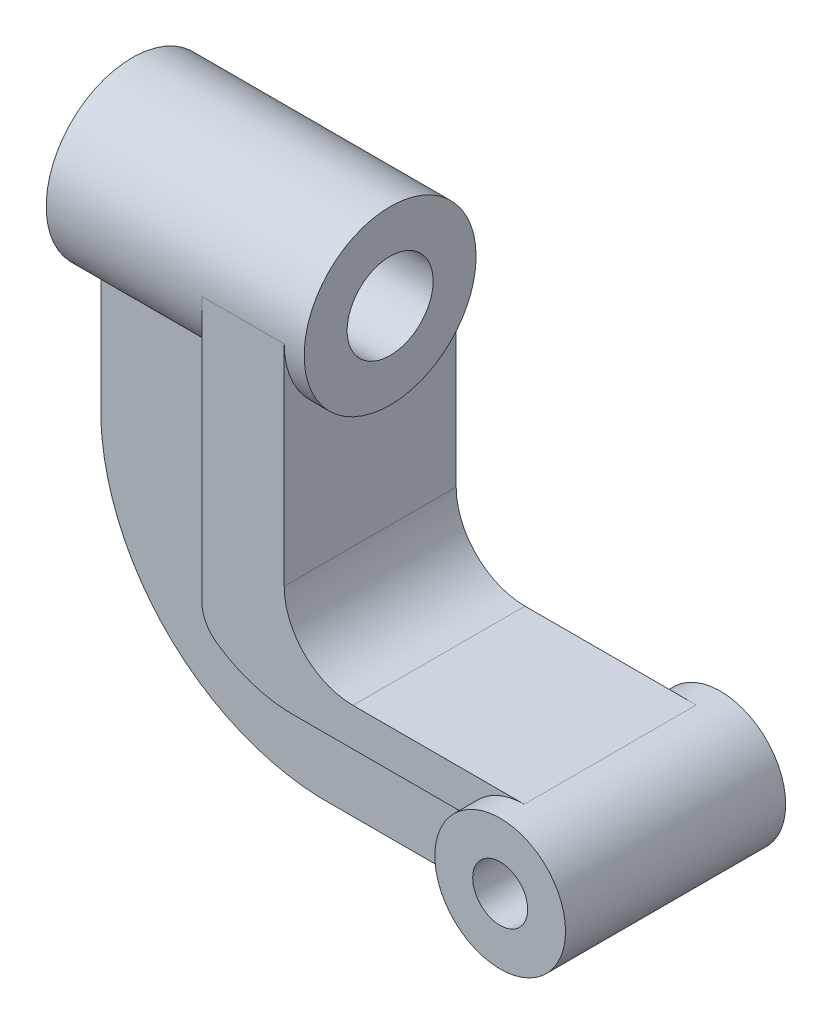
ISO-10303-21;
HEADER;
FILE_DESCRIPTION(('STEP AP214'),'2;1');
FILE_NAME('part.step','',(''),(''),'','','');
FILE_SCHEMA(('AUTOMOTIVE_DESIGN { 1 0 10303 214 1 1 1 1 }'));
ENDSEC;
DATA;
#1=APPLICATION_CONTEXT('core data for automotive mechanical design processes');
#2=APPLICATION_PROTOCOL_DEFINITION('international standard','automotive_design',2000,#1);
#3=PRODUCT_CONTEXT('',#1,'mechanical');
#4=PRODUCT('Part','Part','',(#3));
#5=PRODUCT_RELATED_PRODUCT_CATEGORY('part','',(#4));
#6=PRODUCT_DEFINITION_FORMATION('','',#4);
#7=PRODUCT_DEFINITION_CONTEXT('part definition',#1,'design');
#8=PRODUCT_DEFINITION('design','',#6,#7);
#9=PRODUCT_DEFINITION_SHAPE('','',#8);
#10=(LENGTH_UNIT() NAMED_UNIT(*) SI_UNIT(.MILLI.,.METRE.));
#11=(NAMED_UNIT(*) PLANE_ANGLE_UNIT() SI_UNIT($,.RADIAN.));
#12=(NAMED_UNIT(*) SI_UNIT($,.STERADIAN.) SOLID_ANGLE_UNIT());
#13=UNCERTAINTY_MEASURE_WITH_UNIT(LENGTH_MEASURE(1.E-05),#10,'distance_accuracy_value','');
#14=(GEOMETRIC_REPRESENTATION_CONTEXT(3) GLOBAL_UNCERTAINTY_ASSIGNED_CONTEXT((#13)) GLOBAL_UNIT_ASSIGNED_CONTEXT((#10,
#11,#12)) REPRESENTATION_CONTEXT('',''));
#15=CARTESIAN_POINT('',(0.,0.,0.));
#16=DIRECTION('',(0.,0.,1.));
#17=DIRECTION('',(1.,0.,0.));
#18=AXIS2_PLACEMENT_3D('',#15,#16,#17);
#19=CARTESIAN_POINT('',(37.5,0.,0.));
#20=DIRECTION('',(-1.,0.,0.));
#21=DIRECTION('',(0.,0.,1.));
#22=AXIS2_PLACEMENT_3D('',#19,#20,#21);
#23=CYLINDRICAL_SURFACE('',#22,25.);
#24=CARTESIAN_POINT('',(-37.5,0.,0.));
#25=DIRECTION('',(1.,0.,0.));
#26=DIRECTION('',(0.,0.,-1.));
#27=AXIS2_PLACEMENT_3D('',#24,#25,#26);
#28=CIRCLE('',#27,25.);
#29=CARTESIAN_POINT('',(-37.5,0.,-25.));
#30=VERTEX_POINT('',#29);
#31=EDGE_CURVE('E308',#30,#30,#28,.T.);
#32=ORIENTED_EDGE('',*,*,#31,.T.);
#33=EDGE_LOOP('',(#32));
#34=FACE_BOUND('',#33,.T.);
#35=CARTESIAN_POINT('',(37.5,0.,0.));
#36=DIRECTION('',(1.,0.,0.));
#37=DIRECTION('',(0.,0.,-1.));
#38=AXIS2_PLACEMENT_3D('',#35,#36,#37);
#39=CIRCLE('',#38,25.);
#40=CARTESIAN_POINT('',(37.5,0.,-25.));
#41=VERTEX_POINT('',#40);
#42=EDGE_CURVE('E307',#41,#41,#39,.T.);
#43=ORIENTED_EDGE('',*,*,#42,.F.);
#44=EDGE_LOOP('',(#43));
#45=FACE_BOUND('',#44,.T.);
#46=CARTESIAN_POINT('',(7.76948081400925,0.,0.));
#47=DIRECTION('',(1.,0.,0.));
#48=DIRECTION('',(0.,0.,-1.));
#49=AXIS2_PLACEMENT_3D('',#46,#47,#48);
#50=CIRCLE('',#49,25.);
#51=CARTESIAN_POINT('',(7.76948081400925,0.,25.));
#52=VERTEX_POINT('',#51);
#53=CARTESIAN_POINT('',(7.76948081400925,-20.,15.));
#54=VERTEX_POINT('',#53);
#55=EDGE_CURVE('E65',#52,#54,#50,.T.);
#56=ORIENTED_EDGE('',*,*,#55,.F.);
#57=DIRECTION('',(-1.,0.,0.));
#58=VECTOR('',#57,1.);
#59=CARTESIAN_POINT('',(7.76948081400925,0.,25.));
#60=LINE('',#59,#58);
#61=CARTESIAN_POINT('',(31.7044456882693,0.,25.));
#62=VERTEX_POINT('',#61);
#63=EDGE_CURVE('E67',#62,#52,#60,.T.);
#64=ORIENTED_EDGE('',*,*,#63,.F.);
#65=CARTESIAN_POINT('',(31.7044456882693,0.,0.));
#66=DIRECTION('',(-1.,0.,0.));
#67=DIRECTION('',(0.,0.,1.));
#68=AXIS2_PLACEMENT_3D('',#65,#66,#67);
#69=CIRCLE('',#68,25.);
#70=CARTESIAN_POINT('',(31.7044456882693,0.,-25.));
#71=VERTEX_POINT('',#70);
#72=EDGE_CURVE('E11',#71,#62,#69,.T.);
#73=ORIENTED_EDGE('',*,*,#72,.F.);
#74=DIRECTION('',(-1.,0.,0.));
#75=VECTOR('',#74,1.);
#76=CARTESIAN_POINT('',(7.76948081400925,0.,-25.));
#77=LINE('',#76,#75);
#78=CARTESIAN_POINT('',(7.76948081400925,0.,-25.));
#79=VERTEX_POINT('',#78);
#80=EDGE_CURVE('E177',#71,#79,#77,.T.);
#81=ORIENTED_EDGE('',*,*,#80,.T.);
#82=CARTESIAN_POINT('',(7.76948081400925,-20.,-15.));
#83=VERTEX_POINT('',#82);
#84=EDGE_CURVE('E187',#83,#79,#50,.T.);
#85=ORIENTED_EDGE('',*,*,#84,.F.);
#86=DIRECTION('',(-1.,0.,0.));
#87=VECTOR('',#86,1.);
#88=CARTESIAN_POINT('',(37.5,-20.,-15.));
#89=LINE('',#88,#87);
#90=CARTESIAN_POINT('',(-31.6183252898291,-20.,-15.));
#91=VERTEX_POINT('',#90);
#92=EDGE_CURVE('E309',#91,#83,#89,.F.);
#93=ORIENTED_EDGE('',*,*,#92,.F.);
#94=CARTESIAN_POINT('',(-31.6183252898291,0.,0.));
#95=DIRECTION('',(-1.,0.,0.));
#96=DIRECTION('',(0.,0.,1.));
#97=AXIS2_PLACEMENT_3D('',#94,#95,#96);
#98=CIRCLE('',#97,25.);
#99=CARTESIAN_POINT('',(-31.6183252898291,-20.,15.));
#100=VERTEX_POINT('',#99);
#101=EDGE_CURVE('E312',#91,#100,#98,.T.);
#102=ORIENTED_EDGE('',*,*,#101,.T.);
#103=DIRECTION('',(-1.,0.,0.));
#104=VECTOR('',#103,1.);
#105=CARTESIAN_POINT('',(37.5,-20.,15.));
#106=LINE('',#105,#104);
#107=EDGE_CURVE('E320',#100,#54,#106,.F.);
#108=ORIENTED_EDGE('',*,*,#107,.T.);
#109=EDGE_LOOP('',(#56,#64,#73,#81,#85,#93,#102,#108));
#110=FACE_BOUND('',#109,.T.);
#111=ADVANCED_FACE('F50',(#34,#45,#110),#23,.T.);
#112=CARTESIAN_POINT('',(101.5,-100.,32.));
#113=DIRECTION('',(0.,0.,-1.));
#114=DIRECTION('',(-1.,0.,0.));
#115=AXIS2_PLACEMENT_3D('',#112,#113,#114);
#116=CYLINDRICAL_SURFACE('',#115,19.);
#117=CARTESIAN_POINT('',(101.5,-100.,-32.));
#118=DIRECTION('',(0.,0.,1.));
#119=DIRECTION('',(1.,0.,0.));
#120=AXIS2_PLACEMENT_3D('',#117,#118,#119);
#121=CIRCLE('',#120,19.);
#122=CARTESIAN_POINT('',(120.5,-100.,-32.));
#123=VERTEX_POINT('',#122);
#124=EDGE_CURVE('E260',#123,#123,#121,.T.);
#125=ORIENTED_EDGE('',*,*,#124,.T.);
#126=EDGE_LOOP('',(#125));
#127=FACE_BOUND('',#126,.T.);
#128=CARTESIAN_POINT('',(101.5,-100.,32.));
#129=DIRECTION('',(0.,0.,1.));
#130=DIRECTION('',(1.,0.,0.));
#131=AXIS2_PLACEMENT_3D('',#128,#129,#130);
#132=CIRCLE('',#131,19.);
#133=CARTESIAN_POINT('',(120.5,-100.,32.));
#134=VERTEX_POINT('',#133);
#135=EDGE_CURVE('E251',#134,#134,#132,.T.);
#136=ORIENTED_EDGE('',*,*,#135,.F.);
#137=EDGE_LOOP('',(#136));
#138=FACE_BOUND('',#137,.T.);
#139=DIRECTION('',(0.,0.,-1.));
#140=VECTOR('',#139,1.);
#141=CARTESIAN_POINT('',(84.258248254357,-92.0173941133477,25.));
#142=LINE('',#141,#140);
#143=CARTESIAN_POINT('',(84.258248254357,-92.0173941133477,25.));
#144=VERTEX_POINT('',#143);
#145=CARTESIAN_POINT('',(84.258248254357,-92.0173941133477,15.));
#146=VERTEX_POINT('',#145);
#147=EDGE_CURVE('E243',#144,#146,#142,.T.);
#148=ORIENTED_EDGE('',*,*,#147,.T.);
#149=CARTESIAN_POINT('',(101.5,-100.,15.));
#150=DIRECTION('',(0.,0.,1.));
#151=DIRECTION('',(1.,0.,0.));
#152=AXIS2_PLACEMENT_3D('',#149,#150,#151);
#153=CIRCLE('',#152,19.);
#154=CARTESIAN_POINT('',(101.5,-119.,15.));
#155=VERTEX_POINT('',#154);
#156=EDGE_CURVE('E261',#155,#146,#153,.F.);
#157=ORIENTED_EDGE('',*,*,#156,.F.);
#158=DIRECTION('',(0.,0.,-1.));
#159=VECTOR('',#158,1.);
#160=CARTESIAN_POINT('',(101.5,-119.,15.));
#161=LINE('',#160,#159);
#162=CARTESIAN_POINT('',(101.5,-119.,-15.));
#163=VERTEX_POINT('',#162);
#164=EDGE_CURVE('E283',#155,#163,#161,.T.);
#165=ORIENTED_EDGE('',*,*,#164,.T.);
#166=CARTESIAN_POINT('',(101.5,-100.,-15.));
#167=DIRECTION('',(0.,0.,1.));
#168=DIRECTION('',(1.,0.,0.));
#169=AXIS2_PLACEMENT_3D('',#166,#167,#168);
#170=CIRCLE('',#169,19.);
#171=CARTESIAN_POINT('',(84.258248254357,-92.0173941133477,-15.));
#172=VERTEX_POINT('',#171);
#173=EDGE_CURVE('E258',#163,#172,#170,.F.);
#174=ORIENTED_EDGE('',*,*,#173,.T.);
#175=DIRECTION('',(0.,0.,-1.));
#176=VECTOR('',#175,1.);
#177=CARTESIAN_POINT('',(84.258248254357,-92.0173941133477,32.));
#178=LINE('',#177,#176);
#179=CARTESIAN_POINT('',(84.258248254357,-92.0173941133477,-25.));
#180=VERTEX_POINT('',#179);
#181=EDGE_CURVE('E54',#180,#172,#178,.F.);
#182=ORIENTED_EDGE('',*,*,#181,.F.);
#183=CARTESIAN_POINT('',(101.5,-100.,-25.));
#184=DIRECTION('',(0.,0.,-1.));
#185=DIRECTION('',(-1.,0.,0.));
#186=AXIS2_PLACEMENT_3D('',#183,#184,#185);
#187=CIRCLE('',#186,19.);
#188=CARTESIAN_POINT('',(101.5,-81.,-25.));
#189=VERTEX_POINT('',#188);
#190=EDGE_CURVE('E221',#180,#189,#187,.T.);
#191=ORIENTED_EDGE('',*,*,#190,.T.);
#192=DIRECTION('',(0.,0.,-1.));
#193=VECTOR('',#192,1.);
#194=CARTESIAN_POINT('',(101.5,-81.,25.));
#195=LINE('',#194,#193);
#196=CARTESIAN_POINT('',(101.5,-81.,25.));
#197=VERTEX_POINT('',#196);
#198=EDGE_CURVE('E238',#197,#189,#195,.T.);
#199=ORIENTED_EDGE('',*,*,#198,.F.);
#200=CARTESIAN_POINT('',(101.5,-100.,25.));
#201=DIRECTION('',(0.,0.,-1.));
#202=DIRECTION('',(-1.,0.,0.));
#203=AXIS2_PLACEMENT_3D('',#200,#201,#202);
#204=CIRCLE('',#203,19.);
#205=EDGE_CURVE('E203',#144,#197,#204,.T.);
#206=ORIENTED_EDGE('',*,*,#205,.F.);
#207=EDGE_LOOP('',(#148,#157,#165,#174,#182,#191,#199,#206));
#208=FACE_BOUND('',#207,.T.);
#209=ADVANCED_FACE('F330',(#127,#138,#208),#116,.T.);
#210=CARTESIAN_POINT('',(37.5,0.,0.));
#211=DIRECTION('',(1.,0.,0.));
#212=DIRECTION('',(0.,0.,-1.));
#213=AXIS2_PLACEMENT_3D('',#210,#211,#212);
#214=PLANE('',#213);
#215=CARTESIAN_POINT('',(37.5,0.,0.));
#216=DIRECTION('',(1.,0.,0.));
#217=DIRECTION('',(0.,0.,-1.));
#218=AXIS2_PLACEMENT_3D('',#215,#216,#217);
#219=CIRCLE('',#218,12.5);
#220=CARTESIAN_POINT('',(37.5,0.,-12.5));
#221=VERTEX_POINT('',#220);
#222=EDGE_CURVE('E784',#221,#221,#219,.T.);
#223=ORIENTED_EDGE('',*,*,#222,.F.);
#224=EDGE_LOOP('',(#223));
#225=FACE_BOUND('',#224,.T.);
#226=ORIENTED_EDGE('',*,*,#42,.T.);
#227=EDGE_LOOP('',(#226));
#228=FACE_BOUND('',#227,.T.);
#229=ADVANCED_FACE('F399',(#225,#228),#214,.T.);
#230=CARTESIAN_POINT('',(-37.5,0.,0.));
#231=DIRECTION('',(1.,0.,0.));
#232=DIRECTION('',(0.,0.,-1.));
#233=AXIS2_PLACEMENT_3D('',#230,#231,#232);
#234=PLANE('',#233);
#235=CARTESIAN_POINT('',(-37.5,0.,0.));
#236=DIRECTION('',(1.,0.,0.));
#237=DIRECTION('',(0.,0.,-1.));
#238=AXIS2_PLACEMENT_3D('',#235,#236,#237);
#239=CIRCLE('',#238,12.5);
#240=CARTESIAN_POINT('',(-37.5,0.,-12.5));
#241=VERTEX_POINT('',#240);
#242=EDGE_CURVE('E49',#241,#241,#239,.T.);
#243=ORIENTED_EDGE('',*,*,#242,.T.);
#244=EDGE_LOOP('',(#243));
#245=FACE_BOUND('',#244,.T.);
#246=ORIENTED_EDGE('',*,*,#31,.F.);
#247=EDGE_LOOP('',(#246));
#248=FACE_BOUND('',#247,.T.);
#249=ADVANCED_FACE('F410',(#245,#248),#234,.F.);
#250=CARTESIAN_POINT('',(0.,0.,15.));
#251=DIRECTION('',(0.,0.,1.));
#252=DIRECTION('',(1.,0.,0.));
#253=AXIS2_PLACEMENT_3D('',#250,#251,#252);
#254=PLANE('',#253);
#255=DIRECTION('',(-1.,0.,0.));
#256=VECTOR('',#255,1.);
#257=CARTESIAN_POINT('',(0.,-119.,15.));
#258=LINE('',#257,#256);
#259=CARTESIAN_POINT('',(36.7078458502045,-119.,15.));
#260=VERTEX_POINT('',#259);
#261=EDGE_CURVE('E274',#155,#260,#258,.T.);
#262=ORIENTED_EDGE('',*,*,#261,.F.);
#263=ORIENTED_EDGE('',*,*,#156,.T.);
#264=DIRECTION('',(1.,0.,0.));
#265=VECTOR('',#264,1.);
#266=CARTESIAN_POINT('',(0.,-92.0173941133477,15.));
#267=LINE('',#266,#265);
#268=CARTESIAN_POINT('',(35.7388362704793,-92.0173941133477,15.));
#269=VERTEX_POINT('',#268);
#270=EDGE_CURVE('E279',#269,#146,#267,.T.);
#271=ORIENTED_EDGE('',*,*,#270,.F.);
#272=CARTESIAN_POINT('',(34.3391557664318,-53.0425189437389,15.));
#273=DIRECTION('',(0.,0.,1.));
#274=DIRECTION('',(1.,0.,0.));
#275=AXIS2_PLACEMENT_3D('',#272,#273,#274);
#276=CIRCLE('',#275,39.);
#277=CARTESIAN_POINT('',(12.0557997959325,-85.0495813939547,15.));
#278=VERTEX_POINT('',#277);
#279=EDGE_CURVE('E282',#269,#278,#276,.F.);
#280=ORIENTED_EDGE('',*,*,#279,.T.);
#281=CARTESIAN_POINT('',(17.7694808140093,-76.8426423041558,15.));
#282=DIRECTION('',(0.,0.,1.));
#283=DIRECTION('',(1.,0.,0.));
#284=AXIS2_PLACEMENT_3D('',#281,#282,#283);
#285=CIRCLE('',#284,10.);
#286=CARTESIAN_POINT('',(7.76948081400925,-76.8426423041558,15.));
#287=VERTEX_POINT('',#286);
#288=EDGE_CURVE('E264',#287,#278,#285,.T.);
#289=ORIENTED_EDGE('',*,*,#288,.F.);
#290=DIRECTION('',(0.,-1.,0.));
#291=VECTOR('',#290,1.);
#292=CARTESIAN_POINT('',(7.76948081400925,0.,15.));
#293=LINE('',#292,#291);
#294=EDGE_CURVE('E181',#54,#287,#293,.T.);
#295=ORIENTED_EDGE('',*,*,#294,.F.);
#296=ORIENTED_EDGE('',*,*,#107,.F.);
#297=DIRECTION('',(0.,1.,0.));
#298=VECTOR('',#297,1.);
#299=CARTESIAN_POINT('',(-31.6183252898291,0.,15.));
#300=LINE('',#299,#298);
#301=CARTESIAN_POINT('',(-31.6183252898291,-55.4112090275135,15.));
#302=VERTEX_POINT('',#301);
#303=EDGE_CURVE('E267',#302,#100,#300,.T.);
#304=ORIENTED_EDGE('',*,*,#303,.F.);
#305=CARTESIAN_POINT('',(34.3391557664318,-53.0425189437389,15.));
#306=DIRECTION('',(0.,0.,1.));
#307=DIRECTION('',(1.,0.,0.));
#308=AXIS2_PLACEMENT_3D('',#305,#306,#307);
#309=CIRCLE('',#308,66.);
#310=EDGE_CURVE('E275',#260,#302,#309,.F.);
#311=ORIENTED_EDGE('',*,*,#310,.F.);
#312=EDGE_LOOP('',(#262,#263,#271,#280,#289,#295,#296,#304,#311));
#313=FACE_BOUND('',#312,.T.);
#314=ADVANCED_FACE('F363',(#313),#254,.T.);
#315=CARTESIAN_POINT('',(0.,0.,-15.));
#316=DIRECTION('',(0.,0.,1.));
#317=DIRECTION('',(1.,0.,0.));
#318=AXIS2_PLACEMENT_3D('',#315,#316,#317);
#319=PLANE('',#318);
#320=ORIENTED_EDGE('',*,*,#173,.F.);
#321=DIRECTION('',(-1.,0.,0.));
#322=VECTOR('',#321,1.);
#323=CARTESIAN_POINT('',(0.,-119.,-15.));
#324=LINE('',#323,#322);
#325=CARTESIAN_POINT('',(36.7078458502045,-119.,-15.));
#326=VERTEX_POINT('',#325);
#327=EDGE_CURVE('E291',#163,#326,#324,.T.);
#328=ORIENTED_EDGE('',*,*,#327,.T.);
#329=CARTESIAN_POINT('',(34.3391557664318,-53.0425189437389,-15.));
#330=DIRECTION('',(0.,0.,1.));
#331=DIRECTION('',(1.,0.,0.));
#332=AXIS2_PLACEMENT_3D('',#329,#330,#331);
#333=CIRCLE('',#332,66.);
#334=CARTESIAN_POINT('',(-31.6183252898291,-55.4112090275135,-15.));
#335=VERTEX_POINT('',#334);
#336=EDGE_CURVE('E286',#326,#335,#333,.F.);
#337=ORIENTED_EDGE('',*,*,#336,.T.);
#338=DIRECTION('',(0.,1.,0.));
#339=VECTOR('',#338,1.);
#340=CARTESIAN_POINT('',(-31.6183252898291,0.,-15.));
#341=LINE('',#340,#339);
#342=EDGE_CURVE('E290',#335,#91,#341,.T.);
#343=ORIENTED_EDGE('',*,*,#342,.T.);
#344=ORIENTED_EDGE('',*,*,#92,.T.);
#345=DIRECTION('',(0.,-1.,0.));
#346=VECTOR('',#345,1.);
#347=CARTESIAN_POINT('',(7.76948081400925,0.,-15.));
#348=LINE('',#347,#346);
#349=CARTESIAN_POINT('',(7.76948081400925,-76.8426423041558,-15.));
#350=VERTEX_POINT('',#349);
#351=EDGE_CURVE('E281',#83,#350,#348,.T.);
#352=ORIENTED_EDGE('',*,*,#351,.T.);
#353=CARTESIAN_POINT('',(17.7694808140093,-76.8426423041558,-15.));
#354=DIRECTION('',(0.,0.,1.));
#355=DIRECTION('',(1.,0.,0.));
#356=AXIS2_PLACEMENT_3D('',#353,#354,#355);
#357=CIRCLE('',#356,10.);
#358=CARTESIAN_POINT('',(12.0557997959325,-85.0495813939547,-15.));
#359=VERTEX_POINT('',#358);
#360=EDGE_CURVE('E262',#350,#359,#357,.T.);
#361=ORIENTED_EDGE('',*,*,#360,.T.);
#362=CARTESIAN_POINT('',(34.3391557664318,-53.0425189437389,-15.));
#363=DIRECTION('',(0.,0.,1.));
#364=DIRECTION('',(1.,0.,0.));
#365=AXIS2_PLACEMENT_3D('',#362,#363,#364);
#366=CIRCLE('',#365,39.);
#367=CARTESIAN_POINT('',(35.7388362704793,-92.0173941133477,-15.));
#368=VERTEX_POINT('',#367);
#369=EDGE_CURVE('E270',#368,#359,#366,.F.);
#370=ORIENTED_EDGE('',*,*,#369,.F.);
#371=DIRECTION('',(1.,0.,0.));
#372=VECTOR('',#371,1.);
#373=CARTESIAN_POINT('',(0.,-92.0173941133477,-15.));
#374=LINE('',#373,#372);
#375=EDGE_CURVE('E297',#368,#172,#374,.T.);
#376=ORIENTED_EDGE('',*,*,#375,.T.);
#377=EDGE_LOOP('',(#320,#328,#337,#343,#344,#352,#361,#370,#376));
#378=FACE_BOUND('',#377,.T.);
#379=ADVANCED_FACE('F335',(#378),#319,.F.);
#380=CARTESIAN_POINT('',(-31.6183252898291,0.,15.));
#381=DIRECTION('',(-1.,0.,0.));
#382=DIRECTION('',(0.,0.,1.));
#383=AXIS2_PLACEMENT_3D('',#380,#381,#382);
#384=PLANE('',#383);
#385=ORIENTED_EDGE('',*,*,#101,.F.);
#386=ORIENTED_EDGE('',*,*,#342,.F.);
#387=DIRECTION('',(0.,0.,-1.));
#388=VECTOR('',#387,1.);
#389=CARTESIAN_POINT('',(-31.6183252898291,-55.4112090275135,15.));
#390=LINE('',#389,#388);
#391=EDGE_CURVE('E304',#302,#335,#390,.T.);
#392=ORIENTED_EDGE('',*,*,#391,.F.);
#393=ORIENTED_EDGE('',*,*,#303,.T.);
#394=EDGE_LOOP('',(#385,#386,#392,#393));
#395=FACE_BOUND('',#394,.T.);
#396=ADVANCED_FACE('F375',(#395),#384,.T.);
#397=CARTESIAN_POINT('',(34.3391557664318,-53.0425189437389,15.));
#398=DIRECTION('',(0.,0.,-1.));
#399=DIRECTION('',(-1.,0.,0.));
#400=AXIS2_PLACEMENT_3D('',#397,#398,#399);
#401=CYLINDRICAL_SURFACE('',#400,66.);
#402=ORIENTED_EDGE('',*,*,#336,.F.);
#403=DIRECTION('',(0.,0.,-1.));
#404=VECTOR('',#403,1.);
#405=CARTESIAN_POINT('',(36.7078458502045,-119.,15.));
#406=LINE('',#405,#404);
#407=EDGE_CURVE('E305',#260,#326,#406,.T.);
#408=ORIENTED_EDGE('',*,*,#407,.F.);
#409=ORIENTED_EDGE('',*,*,#310,.T.);
#410=ORIENTED_EDGE('',*,*,#391,.T.);
#411=EDGE_LOOP('',(#402,#408,#409,#410));
#412=FACE_BOUND('',#411,.T.);
#413=ADVANCED_FACE('F376',(#412),#401,.T.);
#414=CARTESIAN_POINT('',(0.,-119.,15.));
#415=DIRECTION('',(0.,-1.,0.));
#416=DIRECTION('',(0.,0.,-1.));
#417=AXIS2_PLACEMENT_3D('',#414,#415,#416);
#418=PLANE('',#417);
#419=ORIENTED_EDGE('',*,*,#327,.F.);
#420=ORIENTED_EDGE('',*,*,#164,.F.);
#421=ORIENTED_EDGE('',*,*,#261,.T.);
#422=ORIENTED_EDGE('',*,*,#407,.T.);
#423=EDGE_LOOP('',(#419,#420,#421,#422));
#424=FACE_BOUND('',#423,.T.);
#425=ADVANCED_FACE('F378',(#424),#418,.T.);
#426=CARTESIAN_POINT('',(0.,0.,32.));
#427=DIRECTION('',(0.,0.,1.));
#428=DIRECTION('',(1.,0.,0.));
#429=AXIS2_PLACEMENT_3D('',#426,#427,#428);
#430=PLANE('',#429);
#431=CARTESIAN_POINT('',(101.5,-100.,32.));
#432=DIRECTION('',(0.,0.,1.));
#433=DIRECTION('',(1.,0.,0.));
#434=AXIS2_PLACEMENT_3D('',#431,#432,#433);
#435=CIRCLE('',#434,8.00000000000001);
#436=CARTESIAN_POINT('',(109.5,-100.,32.));
#437=VERTEX_POINT('',#436);
#438=EDGE_CURVE('E779',#437,#437,#435,.T.);
#439=ORIENTED_EDGE('',*,*,#438,.F.);
#440=EDGE_LOOP('',(#439));
#441=FACE_BOUND('',#440,.T.);
#442=ORIENTED_EDGE('',*,*,#135,.T.);
#443=EDGE_LOOP('',(#442));
#444=FACE_BOUND('',#443,.T.);
#445=ADVANCED_FACE('F425',(#441,#444),#430,.T.);
#446=CARTESIAN_POINT('',(0.,0.,-32.));
#447=DIRECTION('',(0.,0.,1.));
#448=DIRECTION('',(1.,0.,0.));
#449=AXIS2_PLACEMENT_3D('',#446,#447,#448);
#450=PLANE('',#449);
#451=CARTESIAN_POINT('',(101.5,-100.,-32.));
#452=DIRECTION('',(0.,0.,-1.));
#453=DIRECTION('',(-1.,0.,0.));
#454=AXIS2_PLACEMENT_3D('',#451,#452,#453);
#455=CIRCLE('',#454,8.00000000000001);
#456=CARTESIAN_POINT('',(93.5,-100.,-32.));
#457=VERTEX_POINT('',#456);
#458=EDGE_CURVE('E785',#457,#457,#455,.T.);
#459=ORIENTED_EDGE('',*,*,#458,.F.);
#460=EDGE_LOOP('',(#459));
#461=FACE_BOUND('',#460,.T.);
#462=ORIENTED_EDGE('',*,*,#124,.F.);
#463=EDGE_LOOP('',(#462));
#464=FACE_BOUND('',#463,.T.);
#465=ADVANCED_FACE('F430',(#461,#464),#450,.F.);
#466=CARTESIAN_POINT('',(7.76948081400925,-20.,25.));
#467=DIRECTION('',(1.,0.,0.));
#468=DIRECTION('',(0.,0.,-1.));
#469=AXIS2_PLACEMENT_3D('',#466,#467,#468);
#470=PLANE('',#469);
#471=DIRECTION('',(0.,-1.,0.));
#472=VECTOR('',#471,1.);
#473=CARTESIAN_POINT('',(7.76948081400925,-20.,25.));
#474=LINE('',#473,#472);
#475=CARTESIAN_POINT('',(7.76948081400925,-76.8426423041558,25.));
#476=VERTEX_POINT('',#475);
#477=EDGE_CURVE('E169',#52,#476,#474,.T.);
#478=ORIENTED_EDGE('',*,*,#477,.F.);
#479=ORIENTED_EDGE('',*,*,#55,.T.);
#480=ORIENTED_EDGE('',*,*,#294,.T.);
#481=DIRECTION('',(0.,0.,-1.));
#482=VECTOR('',#481,1.);
#483=CARTESIAN_POINT('',(7.76948081400925,-76.8426423041558,25.));
#484=LINE('',#483,#482);
#485=EDGE_CURVE('E176',#476,#287,#484,.T.);
#486=ORIENTED_EDGE('',*,*,#485,.F.);
#487=EDGE_LOOP('',(#478,#479,#480,#486));
#488=FACE_BOUND('',#487,.T.);
#489=ADVANCED_FACE('F182',(#488),#470,.F.);
#490=ORIENTED_EDGE('',*,*,#351,.F.);
#491=ORIENTED_EDGE('',*,*,#84,.T.);
#492=DIRECTION('',(0.,-1.,0.));
#493=VECTOR('',#492,1.);
#494=CARTESIAN_POINT('',(7.76948081400925,-20.,-25.));
#495=LINE('',#494,#493);
#496=CARTESIAN_POINT('',(7.76948081400925,-76.8426423041558,-25.));
#497=VERTEX_POINT('',#496);
#498=EDGE_CURVE('E215',#79,#497,#495,.T.);
#499=ORIENTED_EDGE('',*,*,#498,.T.);
#500=EDGE_CURVE('E190',#350,#497,#484,.T.);
#501=ORIENTED_EDGE('',*,*,#500,.F.);
#502=EDGE_LOOP('',(#490,#491,#499,#501));
#503=FACE_BOUND('',#502,.T.);
#504=ADVANCED_FACE('F381',(#503),#470,.F.);
#505=CARTESIAN_POINT('',(34.3391557664318,-53.0425189437391,25.));
#506=DIRECTION('',(0.,0.,-1.));
#507=DIRECTION('',(-1.,0.,0.));
#508=AXIS2_PLACEMENT_3D('',#505,#506,#507);
#509=CYLINDRICAL_SURFACE('',#508,38.9999999999999);
#510=DIRECTION('',(0.,0.,-1.));
#511=VECTOR('',#510,1.);
#512=CARTESIAN_POINT('',(35.7388362704793,-92.0173941133477,25.));
#513=LINE('',#512,#511);
#514=CARTESIAN_POINT('',(35.7388362704793,-92.0173941133477,-25.));
#515=VERTEX_POINT('',#514);
#516=EDGE_CURVE('E241',#368,#515,#513,.T.);
#517=ORIENTED_EDGE('',*,*,#516,.F.);
#518=ORIENTED_EDGE('',*,*,#369,.T.);
#519=DIRECTION('',(0.,0.,-1.));
#520=VECTOR('',#519,1.);
#521=CARTESIAN_POINT('',(12.0557997959325,-85.0495813939547,25.));
#522=LINE('',#521,#520);
#523=CARTESIAN_POINT('',(12.0557997959325,-85.0495813939547,-25.));
#524=VERTEX_POINT('',#523);
#525=EDGE_CURVE('E249',#359,#524,#522,.T.);
#526=ORIENTED_EDGE('',*,*,#525,.T.);
#527=CARTESIAN_POINT('',(34.3391557664318,-53.0425189437391,-25.));
#528=DIRECTION('',(0.,0.,1.));
#529=DIRECTION('',(1.,0.,0.));
#530=AXIS2_PLACEMENT_3D('',#527,#528,#529);
#531=CIRCLE('',#530,38.9999999999999);
#532=EDGE_CURVE('E217',#524,#515,#531,.T.);
#533=ORIENTED_EDGE('',*,*,#532,.T.);
#534=EDGE_LOOP('',(#517,#518,#526,#533));
#535=FACE_BOUND('',#534,.T.);
#536=ADVANCED_FACE('F337',(#535),#509,.T.);
#537=CARTESIAN_POINT('',(17.7694808140093,-76.8426423041557,25.));
#538=DIRECTION('',(0.,0.,-1.));
#539=DIRECTION('',(-1.,0.,0.));
#540=AXIS2_PLACEMENT_3D('',#537,#538,#539);
#541=CYLINDRICAL_SURFACE('',#540,10.0000000000001);
#542=ORIENTED_EDGE('',*,*,#525,.F.);
#543=ORIENTED_EDGE('',*,*,#360,.F.);
#544=ORIENTED_EDGE('',*,*,#500,.T.);
#545=CARTESIAN_POINT('',(17.7694808140093,-76.8426423041557,-25.));
#546=DIRECTION('',(0.,0.,1.));
#547=DIRECTION('',(1.,0.,0.));
#548=AXIS2_PLACEMENT_3D('',#545,#546,#547);
#549=CIRCLE('',#548,10.0000000000001);
#550=EDGE_CURVE('E214',#497,#524,#549,.T.);
#551=ORIENTED_EDGE('',*,*,#550,.T.);
#552=EDGE_LOOP('',(#542,#543,#544,#551));
#553=FACE_BOUND('',#552,.T.);
#554=ADVANCED_FACE('F338',(#553),#541,.T.);
#555=CARTESIAN_POINT('',(35.7388362704793,-92.0173941133477,25.));
#556=DIRECTION('',(0.,1.,0.));
#557=DIRECTION('',(0.,0.,1.));
#558=AXIS2_PLACEMENT_3D('',#555,#556,#557);
#559=PLANE('',#558);
#560=ORIENTED_EDGE('',*,*,#181,.T.);
#561=ORIENTED_EDGE('',*,*,#375,.F.);
#562=ORIENTED_EDGE('',*,*,#516,.T.);
#563=DIRECTION('',(1.,0.,0.));
#564=VECTOR('',#563,1.);
#565=CARTESIAN_POINT('',(35.7388362704793,-92.0173941133477,-25.));
#566=LINE('',#565,#564);
#567=EDGE_CURVE('E222',#515,#180,#566,.T.);
#568=ORIENTED_EDGE('',*,*,#567,.T.);
#569=EDGE_LOOP('',(#560,#561,#562,#568));
#570=FACE_BOUND('',#569,.T.);
#571=ADVANCED_FACE('F325',(#570),#559,.F.);
#572=ORIENTED_EDGE('',*,*,#288,.T.);
#573=CARTESIAN_POINT('',(12.0557997959325,-85.0495813939547,25.));
#574=VERTEX_POINT('',#573);
#575=EDGE_CURVE('E192',#574,#278,#522,.T.);
#576=ORIENTED_EDGE('',*,*,#575,.F.);
#577=CARTESIAN_POINT('',(17.7694808140093,-76.8426423041557,25.));
#578=DIRECTION('',(0.,0.,1.));
#579=DIRECTION('',(1.,0.,0.));
#580=AXIS2_PLACEMENT_3D('',#577,#578,#579);
#581=CIRCLE('',#580,10.0000000000001);
#582=EDGE_CURVE('E175',#476,#574,#581,.T.);
#583=ORIENTED_EDGE('',*,*,#582,.F.);
#584=ORIENTED_EDGE('',*,*,#485,.T.);
#585=EDGE_LOOP('',(#572,#576,#583,#584));
#586=FACE_BOUND('',#585,.T.);
#587=ADVANCED_FACE('F189',(#586),#541,.T.);
#588=ORIENTED_EDGE('',*,*,#279,.F.);
#589=CARTESIAN_POINT('',(35.7388362704793,-92.0173941133477,25.));
#590=VERTEX_POINT('',#589);
#591=EDGE_CURVE('E247',#590,#269,#513,.T.);
#592=ORIENTED_EDGE('',*,*,#591,.F.);
#593=CARTESIAN_POINT('',(34.3391557664318,-53.0425189437391,25.));
#594=DIRECTION('',(0.,0.,1.));
#595=DIRECTION('',(1.,0.,0.));
#596=AXIS2_PLACEMENT_3D('',#593,#594,#595);
#597=CIRCLE('',#596,38.9999999999999);
#598=EDGE_CURVE('E193',#574,#590,#597,.T.);
#599=ORIENTED_EDGE('',*,*,#598,.F.);
#600=ORIENTED_EDGE('',*,*,#575,.T.);
#601=EDGE_LOOP('',(#588,#592,#599,#600));
#602=FACE_BOUND('',#601,.T.);
#603=ADVANCED_FACE('F370',(#602),#509,.T.);
#604=ORIENTED_EDGE('',*,*,#270,.T.);
#605=ORIENTED_EDGE('',*,*,#147,.F.);
#606=DIRECTION('',(1.,0.,0.));
#607=VECTOR('',#606,1.);
#608=CARTESIAN_POINT('',(35.7388362704793,-92.0173941133477,25.));
#609=LINE('',#608,#607);
#610=EDGE_CURVE('E191',#590,#144,#609,.T.);
#611=ORIENTED_EDGE('',*,*,#610,.F.);
#612=ORIENTED_EDGE('',*,*,#591,.T.);
#613=EDGE_LOOP('',(#604,#605,#611,#612));
#614=FACE_BOUND('',#613,.T.);
#615=ADVANCED_FACE('F365',(#614),#559,.F.);
#616=CARTESIAN_POINT('',(51.7044456882694,-81.,25.));
#617=DIRECTION('',(0.,-1.,0.));
#618=DIRECTION('',(0.,0.,-1.));
#619=AXIS2_PLACEMENT_3D('',#616,#617,#618);
#620=PLANE('',#619);
#621=DIRECTION('',(-1.,0.,0.));
#622=VECTOR('',#621,1.);
#623=CARTESIAN_POINT('',(51.7044456882694,-81.,-25.));
#624=LINE('',#623,#622);
#625=CARTESIAN_POINT('',(51.7044456882694,-81.,-25.));
#626=VERTEX_POINT('',#625);
#627=EDGE_CURVE('E227',#189,#626,#624,.T.);
#628=ORIENTED_EDGE('',*,*,#627,.T.);
#629=DIRECTION('',(0.,0.,-1.));
#630=VECTOR('',#629,1.);
#631=CARTESIAN_POINT('',(51.7044456882694,-81.,25.));
#632=LINE('',#631,#630);
#633=CARTESIAN_POINT('',(51.7044456882694,-81.,25.));
#634=VERTEX_POINT('',#633);
#635=EDGE_CURVE('E240',#634,#626,#632,.T.);
#636=ORIENTED_EDGE('',*,*,#635,.F.);
#637=DIRECTION('',(-1.,0.,0.));
#638=VECTOR('',#637,1.);
#639=CARTESIAN_POINT('',(51.7044456882694,-81.,25.));
#640=LINE('',#639,#638);
#641=EDGE_CURVE('E204',#197,#634,#640,.T.);
#642=ORIENTED_EDGE('',*,*,#641,.F.);
#643=ORIENTED_EDGE('',*,*,#198,.T.);
#644=EDGE_LOOP('',(#628,#636,#642,#643));
#645=FACE_BOUND('',#644,.T.);
#646=ADVANCED_FACE('F349',(#645),#620,.F.);
#647=CARTESIAN_POINT('',(51.7044456882693,-61.,25.));
#648=DIRECTION('',(0.,0.,-1.));
#649=DIRECTION('',(-1.,0.,0.));
#650=AXIS2_PLACEMENT_3D('',#647,#648,#649);
#651=CYLINDRICAL_SURFACE('',#650,20.);
#652=CARTESIAN_POINT('',(51.7044456882693,-61.,-25.));
#653=DIRECTION('',(0.,0.,-1.));
#654=DIRECTION('',(1.,0.,0.));
#655=AXIS2_PLACEMENT_3D('',#652,#653,#654);
#656=CIRCLE('',#655,20.);
#657=CARTESIAN_POINT('',(31.7044456882693,-60.9999999999999,-25.));
#658=VERTEX_POINT('',#657);
#659=EDGE_CURVE('E228',#626,#658,#656,.T.);
#660=ORIENTED_EDGE('',*,*,#659,.T.);
#661=DIRECTION('',(0.,0.,-1.));
#662=VECTOR('',#661,1.);
#663=CARTESIAN_POINT('',(31.7044456882693,-60.9999999999999,25.));
#664=LINE('',#663,#662);
#665=CARTESIAN_POINT('',(31.7044456882693,-60.9999999999999,25.));
#666=VERTEX_POINT('',#665);
#667=EDGE_CURVE('E211',#666,#658,#664,.T.);
#668=ORIENTED_EDGE('',*,*,#667,.F.);
#669=CARTESIAN_POINT('',(51.7044456882693,-61.,25.));
#670=DIRECTION('',(0.,0.,-1.));
#671=DIRECTION('',(1.,0.,0.));
#672=AXIS2_PLACEMENT_3D('',#669,#670,#671);
#673=CIRCLE('',#672,20.);
#674=EDGE_CURVE('E206',#634,#666,#673,.T.);
#675=ORIENTED_EDGE('',*,*,#674,.F.);
#676=ORIENTED_EDGE('',*,*,#635,.T.);
#677=EDGE_LOOP('',(#660,#668,#675,#676));
#678=FACE_BOUND('',#677,.T.);
#679=ADVANCED_FACE('F353',(#678),#651,.F.);
#680=CARTESIAN_POINT('',(31.7044456882693,0.,25.));
#681=DIRECTION('',(-1.,0.,0.));
#682=DIRECTION('',(0.,0.,1.));
#683=AXIS2_PLACEMENT_3D('',#680,#681,#682);
#684=PLANE('',#683);
#685=DIRECTION('',(0.,1.,0.));
#686=VECTOR('',#685,1.);
#687=CARTESIAN_POINT('',(31.7044456882693,0.,-25.));
#688=LINE('',#687,#686);
#689=EDGE_CURVE('E232',#658,#71,#688,.T.);
#690=ORIENTED_EDGE('',*,*,#689,.T.);
#691=ORIENTED_EDGE('',*,*,#72,.T.);
#692=DIRECTION('',(0.,1.,0.));
#693=VECTOR('',#692,1.);
#694=CARTESIAN_POINT('',(31.7044456882693,-20.,25.));
#695=LINE('',#694,#693);
#696=EDGE_CURVE('E208',#666,#62,#695,.T.);
#697=ORIENTED_EDGE('',*,*,#696,.F.);
#698=ORIENTED_EDGE('',*,*,#667,.T.);
#699=EDGE_LOOP('',(#690,#691,#697,#698));
#700=FACE_BOUND('',#699,.T.);
#701=ADVANCED_FACE('F383',(#700),#684,.F.);
#702=CARTESIAN_POINT('',(51.7044456882693,-61.,25.));
#703=DIRECTION('',(0.,0.,1.));
#704=DIRECTION('',(1.,0.,0.));
#705=AXIS2_PLACEMENT_3D('',#702,#703,#704);
#706=PLANE('',#705);
#707=ORIENTED_EDGE('',*,*,#477,.T.);
#708=ORIENTED_EDGE('',*,*,#582,.T.);
#709=ORIENTED_EDGE('',*,*,#598,.T.);
#710=ORIENTED_EDGE('',*,*,#610,.T.);
#711=ORIENTED_EDGE('',*,*,#205,.T.);
#712=ORIENTED_EDGE('',*,*,#641,.T.);
#713=ORIENTED_EDGE('',*,*,#674,.T.);
#714=ORIENTED_EDGE('',*,*,#696,.T.);
#715=ORIENTED_EDGE('',*,*,#63,.T.);
#716=EDGE_LOOP('',(#707,#708,#709,#710,#711,#712,#713,#714,#715));
#717=FACE_BOUND('',#716,.T.);
#718=ADVANCED_FACE('F168',(#717),#706,.T.);
#719=CARTESIAN_POINT('',(51.7044456882693,-61.,-25.));
#720=DIRECTION('',(0.,0.,1.));
#721=DIRECTION('',(1.,0.,0.));
#722=AXIS2_PLACEMENT_3D('',#719,#720,#721);
#723=PLANE('',#722);
#724=ORIENTED_EDGE('',*,*,#498,.F.);
#725=ORIENTED_EDGE('',*,*,#80,.F.);
#726=ORIENTED_EDGE('',*,*,#689,.F.);
#727=ORIENTED_EDGE('',*,*,#659,.F.);
#728=ORIENTED_EDGE('',*,*,#627,.F.);
#729=ORIENTED_EDGE('',*,*,#190,.F.);
#730=ORIENTED_EDGE('',*,*,#567,.F.);
#731=ORIENTED_EDGE('',*,*,#532,.F.);
#732=ORIENTED_EDGE('',*,*,#550,.F.);
#733=EDGE_LOOP('',(#724,#725,#726,#727,#728,#729,#730,#731,#732));
#734=FACE_BOUND('',#733,.T.);
#735=ADVANCED_FACE('F344',(#734),#723,.F.);
#736=CARTESIAN_POINT('',(-50.5,0.,0.));
#737=DIRECTION('',(1.,0.,0.));
#738=DIRECTION('',(0.,0.,-1.));
#739=AXIS2_PLACEMENT_3D('',#736,#737,#738);
#740=CYLINDRICAL_SURFACE('',#739,12.5);
#741=ORIENTED_EDGE('',*,*,#222,.T.);
#742=EDGE_LOOP('',(#741));
#743=FACE_BOUND('',#742,.T.);
#744=ORIENTED_EDGE('',*,*,#242,.F.);
#745=EDGE_LOOP('',(#744));
#746=FACE_BOUND('',#745,.T.);
#747=ADVANCED_FACE('F472',(#743,#746),#740,.F.);
#748=CARTESIAN_POINT('',(101.5,-100.,56.));
#749=DIRECTION('',(0.,0.,-1.));
#750=DIRECTION('',(-1.,0.,0.));
#751=AXIS2_PLACEMENT_3D('',#748,#749,#750);
#752=CYLINDRICAL_SURFACE('',#751,8.00000000000001);
#753=ORIENTED_EDGE('',*,*,#438,.T.);
#754=EDGE_LOOP('',(#753));
#755=FACE_BOUND('',#754,.T.);
#756=ORIENTED_EDGE('',*,*,#458,.T.);
#757=EDGE_LOOP('',(#756));
#758=FACE_BOUND('',#757,.T.);
#759=ADVANCED_FACE('F479',(#755,#758),#752,.F.);
#760=CLOSED_SHELL('',(#111,#209,#229,#249,#314,#379,#396,#413,#425,#445,#465,#489,#504,#536,
#554,#571,#587,#603,#615,#646,#679,#701,#718,#735,#747,#759));
#761=MANIFOLD_SOLID_BREP('B2',#760);
#762=ADVANCED_BREP_SHAPE_REPRESENTATION('',(#18,#761),#14);
#763=SHAPE_DEFINITION_REPRESENTATION(#9,#762);
ENDSEC;
END-ISO-10303-21;
